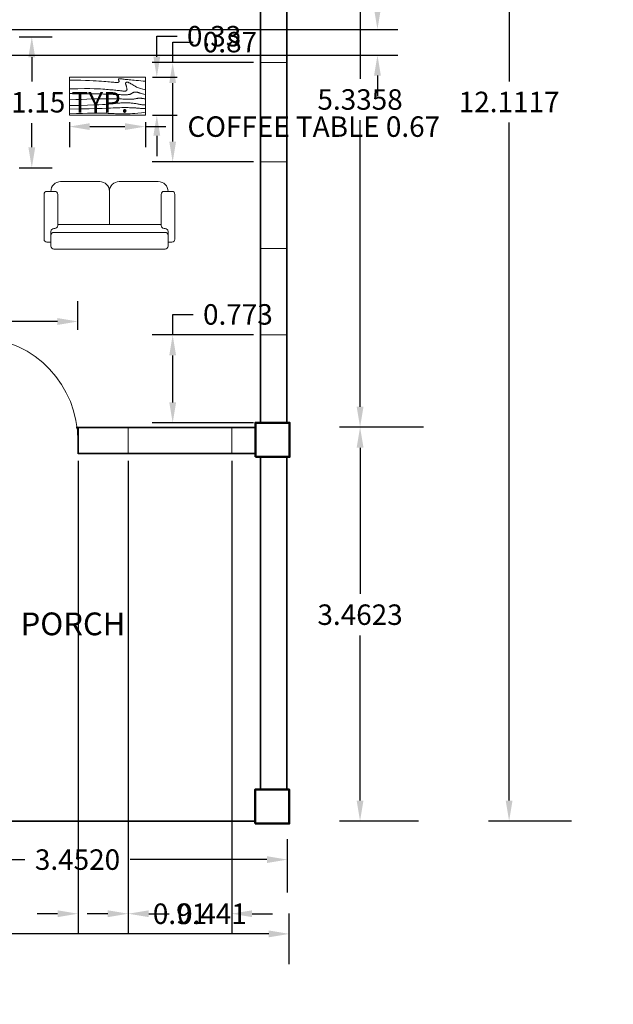
# Model space of a CAD drawing. Units: metres. Extents: x 473.2 to 488.6, y 701.8 to 717.3.
# Tile 3 of 4: x 483.4 to 488.6, y 702.6 to 711.3. Entities that reach past the tile are written whole.
import ezdxf

# ---------------------------------------------------------------- set-up
doc = ezdxf.new("R2010")
doc.units = ezdxf.units.M
doc.header["$PDMODE"] = 32
for name, color, linetype, lineweight in [('A-ANNO-DIMS', 2, 'Continuous', 18), ('A-AREA-IDEN', 7, 'Continuous', 18), ('A-COLS', 7, 'Continuous', 50), ('A-DOOR', 3, 'Continuous', 18), ('A-FURN', 8, 'Continuous', 18), ('A-GLAZ', 4, 'Continuous', 18), ('A-WALL', 7, 'Continuous', 35)]:
    doc.layers.add(name, color=color, linetype=linetype, lineweight=lineweight)
doc.styles.get("Standard").update_dxf_attribs({"font": 'arial.ttf'})
doc.dimstyles.get("Standard").update_dxf_attribs({"dimtxt": 0.18, "dimasz": 0.18, "dimexe": 0.18, "dimexo": 0.0625, "dimgap": 0.09, "dimtad": 0, "dimtih": 1, "dimtoh": 1, "dimdec": 4, "dimzin": 0, "dimdsep": 46, "dimtxsty": 'Standard', "dimcen": 0.09, "dimadec": 0, "dimazin": 0, "dimtfac": 1, "dimtdec": 4, "dimtofl": 0, "dimtmove": 0, "dimatfit": 3, "dimfxl": 1, "dimtolj": 1, "dimtzin": 0, "dimarcsym": 0})

# ---------------------------------------------------------------- blocks, each defined once
blk = doc.blocks.new('A$C02A636C4')
for p, q in [((0.0679, 0.6013), (0.0291, 0.6013)), ((0.0679, 0.6401), (0.0679, 0.6013)), ((0.0679, 0.5334), (0.0679, 0.6013)), ((1.2026, 0.6692), (0.097, 0.6692)), ((1.2317, 0.6401), (1.2317, 0.6013)), ((1.2317, 0.6013), (1.2705, 0.6013)), ((1.2317, 0.5334), (1.2317, 0.6013)), ((0, 0.5722), (0, 0.1261)), ((0.0679, 0.4946), (0.0679, 0.5431)), ((1.2026, 0.5043), (0.097, 0.5043)), ((1.2317, 0.4946), (1.2317, 0.5431)), ((1.2996, 0.5722), (1.2996, 0.1261)), ((0.1067, 0.4655), (0.097, 0.4655)), ((0.1358, 0.1261), (0.1358, 0.4364)), ((1.1638, 0.4267), (0.1358, 0.4267)), ((0.6498, 0.097), (0.6498, 0.4267)), ((1.1638, 0.1261), (1.1638, 0.4364)), ((1.1929, 0.4655), (1.2026, 0.4655)), ((0.0291, 0.097), (0.1067, 0.097)), ((0.1649, 0), (0.5528, 0)), ((0.7468, 0), (1.1347, 0)), ((1.2705, 0.097), (1.1929, 0.097))]:
    blk.add_line(p, q)
for centre, radius, start, end in [((0.0291, 0.5722), 0.0291, 90, 180), ((0.097, 0.6401), 0.0291, 90, 180), ((1.2026, 0.6401), 0.0291, 0, 90), ((1.2705, 0.5722), 0.0291, 0, 90), ((0.097, 0.5334), 0.0291, 180, 270), ((0.097, 0.4946), 0.0291, 180, 270), ((1.2026, 0.5334), 0.0291, 270, 0), ((1.2026, 0.4946), 0.0291, 270, 0), ((0.1067, 0.4364), 0.0291, 0, 90), ((1.1929, 0.4364), 0.0291, 90, 180), ((0.0291, 0.1261), 0.0291, 180, 270), ((0.1067, 0.1261), 0.0291, 270, 0), ((1.1929, 0.1261), 0.0291, 180, 270), ((1.2705, 0.1261), 0.0291, 270, 0), ((0.1649, 0.097), 0.097, 180, 270), ((0.5528, 0.097), 0.097, 270, 0), ((0.7468, 0.097), 0.097, 180, 270), ((1.1347, 0.097), 0.097, 270, 0)]:
    blk.add_arc(centre, radius, start, end)
blk = doc.blocks.new('Table - Rectangular Woodgrain 60 x 30 in.')
for p, q in [((0, 0), (0, -30)), ((60, 0), (0, 0)), ((60, -30), (60, 0)), ((0, -30), (60, -30))]:
    blk.add_line(p, q)
for points in [[(0, -2.4), (4.8155, -2.418), (9.0302, -2.4688), (12.709, -2.5477), (15.9167, -2.65), (18.7181, -2.7711), (21.1781, -2.9063), (23.3616, -3.0508), (25.3333, -3.2), (27.1477, -3.3495), (28.8172, -3.4958), (30.3437, -3.636), (31.7291, -3.7667), (32.9756, -3.8849), (34.0849, -3.9875), (35.059, -4.0714), (35.9, -4.1334), (36.6114, -4.1711), (37.2041, -4.1854), (37.6906, -4.1779), (38.0833, -4.15), (38.3948, -4.1034), (38.6375, -4.0396), (38.8239, -3.9602), (38.9666, -3.8667), (39.0764, -3.7608), (39.1573, -3.6448), (39.2116, -3.521), (39.2416, -3.3917), (39.2498, -3.2593), (39.2385, -3.1261), (39.21, -2.9944), (39.1666, -2.8667), (39.111, -2.7447), (39.0468, -2.6281), (38.978, -2.5163), (38.9083, -2.4083), (38.8418, -2.3035), (38.7823, -2.201), (38.7337, -2.1001), (38.7, -2), (38.6844, -1.9003), (38.6875, -1.8021), (38.7094, -1.707), (38.75, -1.6167), (38.8094, -1.5326), (38.8875, -1.4563), (38.9844, -1.3893), (39.1, -1.3333), (39.2351, -1.2896), (39.3937, -1.2583), (39.5804, -1.2396), (39.8, -1.2333), (40.057, -1.2396), (40.3562, -1.2583), (40.7023, -1.2896), (41.1, -1.3333), (41.5547, -1.3895), (42.0755, -1.4573), (42.6721, -1.5361), (43.3542, -1.625), (44.1316, -1.7233), (45.014, -1.8302), (46.0114, -1.9449), (47.1333, -2.0667), (48.3862, -2.1947), (49.7625, -2.3281), (51.2513, -2.4663), (52.8416, -2.6083), (54.5226, -2.7535), (56.2833, -2.9011), (58.1127, -3.0501), (60, -3.2)], [(0, -9.2), (6.5759, -9.0858), (11.9385, -9.0365), (16.2527, -9.0418), (19.6833, -9.0917), (22.3952, -9.1759), (24.5531, -9.2844), (26.322, -9.4069), (27.8666, -9.5333), (29.3241, -9.6553), (30.7203, -9.7719), (32.0532, -9.8837), (33.3208, -9.9917), (34.5213, -10.0965), (35.6526, -10.199), (36.7128, -10.2999), (37.7, -10.4), (38.6129, -10.4996), (39.4531, -10.5969), (40.223, -10.6895), (40.925, -10.775), (41.5613, -10.8512), (42.1344, -10.9156), (42.6465, -10.966), (43.1, -11), (43.4976, -11.0158), (43.8437, -11.0136), (44.143, -10.9942), (44.4, -10.9583), (44.6195, -10.9069), (44.8062, -10.8406), (44.9648, -10.7603), (45.1, -10.6667), (45.2155, -10.5598), (45.3114, -10.4365), (45.3871, -10.2929), (45.4416, -10.125), (45.4743, -9.929), (45.4844, -9.7011), (45.4709, -9.4371), (45.4333, -9.1333), (45.3716, -8.7883), (45.2896, -8.4104), (45.1919, -8.0107), (45.0833, -7.6), (44.9685, -7.1893), (44.8521, -6.7896), (44.7388, -6.4117), (44.6333, -6.0667), (44.54, -5.7628), (44.4614, -5.4979), (44.4001, -5.2675), (44.3583, -5.0667), (44.3384, -4.8909), (44.3427, -4.7354), (44.3736, -4.5956), (44.4333, -4.4667), (44.5236, -4.3453), (44.6427, -4.2333), (44.7884, -4.1339), (44.9583, -4.05), (45.1501, -3.9849), (45.3614, -3.9417), (45.59, -3.9234), (45.8333, -3.9333), (46.0915, -3.9749), (46.3734, -4.0531), (46.6906, -4.1736), (47.0542, -4.3417), (47.4756, -4.5629), (47.9661, -4.8427), (48.5372, -5.1866), (49.2, -5.6), (49.9676, -6.0844), (50.8594, -6.625), (51.8965, -7.2031), (53.1, -7.8), (54.491, -8.3969), (56.0906, -8.975), (57.9199, -9.5156), (60, -10)], [(0, -12.8), (5.1847, -12.9322), (9.6213, -13.0323), (13.3963, -13.1059), (16.5958, -13.1583), (19.3063, -13.1952), (21.614, -13.2219), (23.6054, -13.2439), (25.3666, -13.2667), (26.9728, -13.2947), (28.4531, -13.3281), (29.8256, -13.3663), (31.1083, -13.4083), (32.3191, -13.4535), (33.476, -13.501), (34.597, -13.5501), (35.7, -13.6), (36.7984, -13.6497), (37.8875, -13.6979), (38.9578, -13.743), (40, -13.7833), (41.0047, -13.8174), (41.9625, -13.8438), (42.864, -13.8607), (43.7, -13.8667), (44.4631, -13.8604), (45.1552, -13.8417), (45.7801, -13.8104), (46.3416, -13.7667), (46.8439, -13.7104), (47.2906, -13.6417), (47.6858, -13.5604), (48.0333, -13.4667), (48.3375, -13.3608), (48.6042, -13.2448), (48.8396, -13.121), (49.05, -12.9917), (49.2417, -12.8593), (49.4208, -12.7261), (49.5937, -12.5944), (49.7667, -12.4667), (49.9452, -12.3451), (50.1323, -12.2313), (50.3303, -12.1268), (50.5416, -12.0333), (50.7686, -11.9524), (51.0135, -11.8854), (51.2788, -11.8341), (51.5666, -11.8), (51.8785, -11.7843), (52.2116, -11.7865), (52.562, -11.8059), (52.926, -11.8417), (53.2998, -11.8931), (53.6795, -11.9594), (54.0614, -12.0397), (54.4416, -12.1333), (54.8223, -12.2401), (55.2293, -12.3625), (55.6942, -12.5037), (56.2489, -12.6667), (56.9251, -12.8547), (57.7545, -13.0708), (58.7689, -13.3182), (60, -13.6)], [(0, -18), (5.124, -17.7273), (9.6609, -17.5057), (13.6705, -17.3303), (17.2125, -17.1958), (20.3467, -17.0973), (23.1328, -17.0297), (25.6307, -16.9878), (27.9, -16.9667), (29.9928, -16.9617), (31.9302, -16.9703), (33.7254, -16.9907), (35.3917, -17.0208), (36.9423, -17.0588), (38.3906, -17.1026), (39.7499, -17.1503), (41.0333, -17.2), (42.2519, -17.2496), (43.4073, -17.2969), (44.4986, -17.3395), (45.525, -17.375), (46.4858, -17.4012), (47.3802, -17.4156), (48.2074, -17.416), (48.9667, -17.4), (49.6583, -17.3662), (50.2872, -17.3167), (50.8595, -17.2547), (51.3812, -17.1833), (51.8584, -17.1057), (52.2971, -17.025), (52.7034, -16.9443), (53.0833, -16.8667), (53.443, -16.7951), (53.789, -16.7313), (54.128, -16.6768), (54.4666, -16.6334), (54.8115, -16.6024), (55.1693, -16.5854), (55.5465, -16.5841), (55.95, -16.6), (56.3828, -16.6337), (56.8346, -16.6823), (57.2915, -16.7418), (57.7396, -16.8084), (58.165, -16.878), (58.5539, -16.9469), (58.8924, -17.0111), (59.1666, -17.0667), (59.3679, -17.1107), (59.5078, -17.1438), (59.6032, -17.1675), (59.6708, -17.1833), (59.7275, -17.193), (59.7901, -17.1979), (59.8753, -17.1998), (60, -17.2)], [(0, -22.4), (8.0098, -22.2501), (14.4094, -22.1011), (19.4168, -21.9535), (23.25, -21.8083), (26.1269, -21.6663), (28.2656, -21.5281), (29.884, -21.3947), (31.2, -21.2667), (32.3967, -21.1448), (33.5172, -21.0292), (34.5697, -20.9198), (35.5625, -20.8167), (36.5037, -20.7198), (37.4015, -20.6292), (38.2642, -20.5448), (39.1, -20.4667), (39.9164, -20.3951), (40.7187, -20.3313), (41.5117, -20.2768), (42.3, -20.2333), (43.0883, -20.2024), (43.8812, -20.1854), (44.6836, -20.1841), (45.5, -20.2), (46.3328, -20.234), (47.1747, -20.2844), (48.0163, -20.3488), (48.8479, -20.425), (49.66, -20.5106), (50.4429, -20.6031), (51.1872, -20.7004), (51.8833, -20.8), (52.5246, -20.8999), (53.1166, -20.9995), (53.6681, -21.0983), (54.1875, -21.1958), (54.6834, -21.2919), (55.1646, -21.3859), (55.6394, -21.4777), (56.1167, -21.5667), (56.6028, -21.6515), (57.0961, -21.7266), (57.5929, -21.7852), (58.0896, -21.8208), (58.5823, -21.8268), (59.0674, -21.7964), (59.5412, -21.723), (60, -21.6)], [(0, -25.2), (8.6355, -25.0504), (15.7026, -24.9031), (21.4049, -24.7606), (25.9458, -24.625), (29.529, -24.4988), (32.3578, -24.3844), (34.6359, -24.284), (36.5667, -24.2), (38.3213, -24.1341), (39.9417, -24.0854), (41.437, -24.0523), (42.8167, -24.0333), (44.0901, -24.0268), (45.2667, -24.0313), (46.3557, -24.0451), (47.3667, -24.0667), (48.309, -24.0947), (49.1928, -24.1287), (50.0284, -24.168), (50.826, -24.2125), (51.5959, -24.2617), (52.3483, -24.3151), (53.0935, -24.3725), (53.8417, -24.4334), (54.6009, -24.497), (55.3699, -24.561), (56.1454, -24.6226), (56.9239, -24.6792), (57.7021, -24.7279), (58.4764, -24.7662), (59.2435, -24.7911), (60, -24.8)], [(0, -28.8), (5.6867, -28.6681), (10.45, -28.5698), (14.407, -28.5012), (17.675, -28.4584), (20.3711, -28.4374), (22.6125, -28.4344), (24.5164, -28.4455), (26.2, -28.4667), (27.762, -28.4947), (29.2276, -28.5281), (30.6033, -28.5663), (31.8958, -28.6084), (33.1118, -28.6535), (34.2578, -28.7011), (35.3405, -28.7501), (36.3666, -28.8), (37.3443, -28.8497), (38.288, -28.8974), (39.2137, -28.9412), (40.1375, -28.9792), (41.0753, -29.0093), (42.0432, -29.0297), (43.0572, -29.0384), (44.1333, -29.0333), (45.2936, -29.0114), (46.5843, -28.9641), (48.0579, -28.8816), (49.7666, -28.7542), (51.7629, -28.5721), (54.0989, -28.3255), (56.8272, -28.0048), (60, -27.6)]]:
    blk.add_lwpolyline(points)
blk = doc.blocks.new('*D14')
at = {"layer": 'A-ANNO-DIMS', "color": 0, "lineweight": -2, "transparency": 16777216}
for p, q in [((486.6804, 713.0126), (486.1829, 713.0126)), ((486.3629, 712.8326), (486.3629, 710.7399)), ((486.3629, 707.8568), (486.3629, 710.376)), ((486.9196, 707.6768), (486.1829, 707.6768))]:
    blk.add_line(p, q, dxfattribs=at)
at = {"layer": 'A-ANNO-DIMS', "color": 0, "transparency": 16777216}
for points in [[(486.3329, 712.8326), (486.3929, 712.8326), (486.3629, 713.0126)], [(486.3329, 707.8568), (486.3929, 707.8568), (486.3629, 707.6768)]]:
    blk.add_solid(points, dxfattribs=at)
at = {"layer": 'Defpoints', "color": 0, "transparency": 16777216}
for p in [(486.3629, 713.0126), (486.7429, 713.0126), (486.9821, 707.6768)]:
    blk.add_point(p, dxfattribs=at)
at = {"layer": 'A-ANNO-DIMS', "color": 0, "transparency": 16777216, "insert": (486.3629, 710.5579), "char_height": 0.18, "width": 1.240263, "attachment_point": 5}
blk.add_mtext('\\A1;5.3358', dxfattribs=at)
blk = doc.blocks.new('*D15')
at = {"layer": 'A-ANNO-DIMS', "color": 0, "lineweight": -2, "transparency": 16777216}
for p, q in [((486.5856, 707.6768), (486.1829, 707.6768)), ((486.3629, 707.4968), (486.3629, 706.2104)), ((486.3629, 704.3946), (486.3629, 705.8465)), ((486.877, 704.2146), (486.1829, 704.2146))]:
    blk.add_line(p, q, dxfattribs=at)
at = {"layer": 'A-ANNO-DIMS', "color": 0, "transparency": 16777216}
for points in [[(486.3329, 707.4968), (486.3929, 707.4968), (486.3629, 707.6768)], [(486.3329, 704.3946), (486.3929, 704.3946), (486.3629, 704.2146)]]:
    blk.add_solid(points, dxfattribs=at)
at = {"layer": 'Defpoints', "color": 0, "transparency": 16777216}
for p in [(486.3629, 707.6768), (486.6481, 707.6768), (486.9395, 704.2146)]:
    blk.add_point(p, dxfattribs=at)
at = {"layer": 'A-ANNO-DIMS', "color": 0, "transparency": 16777216, "insert": (486.3629, 706.0285), "char_height": 0.18, "width": 1.240263, "attachment_point": 5}
blk.add_mtext('\\A1;3.4623', dxfattribs=at)
blk = doc.blocks.new('*D17')
at = {"layer": 'A-ANNO-DIMS', "color": 0, "lineweight": -2, "transparency": 16777216}
for p, q in [((488.5274, 716.3262), (487.4937, 716.3262)), ((487.6737, 716.1462), (487.6737, 710.7165)), ((487.6737, 704.3946), (487.6737, 710.3558)), ((488.2227, 704.2146), (487.4937, 704.2146))]:
    blk.add_line(p, q, dxfattribs=at)
at = {"layer": 'A-ANNO-DIMS', "color": 0, "transparency": 16777216}
for points in [[(487.6437, 716.1462), (487.7037, 716.1462), (487.6737, 716.3262)], [(487.6437, 704.3946), (487.7037, 704.3946), (487.6737, 704.2146)]]:
    blk.add_solid(points, dxfattribs=at)
at = {"layer": 'Defpoints', "color": 0, "transparency": 16777216}
for p in [(487.6737, 716.3262), (488.5899, 716.3262), (488.2852, 704.2146)]:
    blk.add_point(p, dxfattribs=at)
at = {"layer": 'A-ANNO-DIMS', "color": 0, "transparency": 16777216, "insert": (487.6737, 710.5362), "char_height": 0.18, "width": 1.240263, "attachment_point": 5}
blk.add_mtext('\\A1;12.1117', dxfattribs=at)
blk = doc.blocks.new('*D18')
at = {"layer": 'A-ANNO-DIMS', "color": 0, "lineweight": -2, "transparency": 16777216}
for p, q in [((475.798, 702.6656), (475.798, 703.4022)), ((485.74, 702.957), (485.74, 703.4022)), ((475.978, 703.2222), (480.3782, 703.2222)), ((485.56, 703.2222), (481.3049, 703.2222))]:
    blk.add_line(p, q, dxfattribs=at)
at = {"layer": 'A-ANNO-DIMS', "color": 0, "transparency": 16777216}
for points in [[(475.978, 703.2522), (475.978, 703.1922), (475.798, 703.2222)], [(485.56, 703.2522), (485.56, 703.1922), (485.74, 703.2222)]]:
    blk.add_solid(points, dxfattribs=at)
at = {"layer": 'Defpoints', "color": 0, "transparency": 16777216}
for p in [(485.74, 703.2222), (485.74, 702.8945), (475.798, 702.6031)]:
    blk.add_point(p, dxfattribs=at)
at = {"layer": 'A-ANNO-DIMS', "color": 0, "transparency": 16777216, "insert": (480.8416, 703.2222), "char_height": 0.18, "width": 1.240263, "attachment_point": 5}
blk.add_mtext('\\A1;9.9420', dxfattribs=at)
blk = doc.blocks.new('*D21')
at = {"layer": 'A-ANNO-DIMS', "color": 0, "lineweight": -2, "transparency": 16777216}
for p, q in [((482.2714, 703.3187), (482.2714, 704.0553)), ((485.7234, 703.5853), (485.7234, 704.0553)), ((482.4514, 703.8753), (483.415, 703.8753)), ((485.5434, 703.8753), (484.3415, 703.8753))]:
    blk.add_line(p, q, dxfattribs=at)
at = {"layer": 'A-ANNO-DIMS', "color": 0, "transparency": 16777216}
for points in [[(482.4514, 703.9053), (482.4514, 703.8453), (482.2714, 703.8753)], [(485.5434, 703.9053), (485.5434, 703.8453), (485.7234, 703.8753)]]:
    blk.add_solid(points, dxfattribs=at)
at = {"layer": 'Defpoints', "color": 0, "transparency": 16777216}
for p in [(485.7234, 703.8753), (485.7234, 703.5228), (482.2714, 703.2562)]:
    blk.add_point(p, dxfattribs=at)
at = {"layer": 'A-ANNO-DIMS', "color": 0, "transparency": 16777216, "insert": (483.8782, 703.8753), "char_height": 0.18, "width": 1.240263, "attachment_point": 5}
blk.add_mtext('\\A1;3.4520', dxfattribs=at)
blk = doc.blocks.new('DOOR-SWING-910')
for p, q in [((0, 0), (-0.05, 0)), ((-0.05, 0), (-0.05, -0.91)), ((0, 0), (0, -0.91)), ((0, -0.91), (-0.05, -0.91))]:
    blk.add_line(p, q)
blk.add_arc((0.0015, 0), 0.9115, 180, 266.76381)
blk = doc.blocks.new('COL-SQUARE-300')
blk.add_lwpolyline([(-0.15, -0.15), (0.15, -0.15), (0.15, 0.15), (-0.15, 0.15)], close=True)
blk = doc.blocks.new('WIN-1520')
blk.add_line((0.23, 0.76), (0, 0.76))
blk.add_lwpolyline([(0.23, 0), (0.23, 1.52), (0, 1.52), (0, 0)], close=True)
blk = doc.blocks.new('*D27')
at = {"layer": 'A-ANNO-DIMS', "color": 0, "lineweight": -2, "transparency": 16777216}
for p, q in [((482.9717, 708.5321), (482.9717, 708.7861)), ((483.8817, 708.5321), (483.8817, 708.7861)), ((482.9717, 708.6061), (482.7917, 708.6061)), ((483.7017, 708.6061), (483.1517, 708.6061))]:
    blk.add_line(p, q, dxfattribs=at)
at = {"layer": 'A-ANNO-DIMS', "color": 0, "transparency": 16777216}
for points in [[(483.1517, 708.6361), (483.1517, 708.5761), (482.9717, 708.6061)], [(483.7017, 708.6361), (483.7017, 708.5761), (483.8817, 708.6061)]]:
    blk.add_solid(points, dxfattribs=at)
at = {"layer": 'Defpoints', "color": 0, "transparency": 16777216}
for p in [(482.9717, 708.6061), (482.9717, 708.4696), (483.8817, 708.4696)]:
    blk.add_point(p, dxfattribs=at)
at = {"layer": 'A-ANNO-DIMS', "color": 0, "transparency": 16777216, "insert": (481.7511, 708.6061), "char_height": 0.18, "attachment_point": 5}
blk.add_mtext('\\A1;DOOR 0.91 TYP.', dxfattribs=at)
blk = doc.blocks.new('*D33')
at = {"layer": 'A-ANNO-DIMS', "color": 0, "lineweight": -2, "transparency": 16777216}
for p, q in [((483.3662, 711.1086), (483.6562, 711.1086)), ((483.4762, 710.9286), (483.4762, 710.7165)), ((483.4762, 710.1382), (483.4762, 710.3503)), ((483.3662, 709.9582), (483.6562, 709.9582))]:
    blk.add_line(p, q, dxfattribs=at)
at = {"layer": 'A-ANNO-DIMS', "color": 0, "transparency": 16777216}
for points in [[(483.4462, 710.9286), (483.5062, 710.9286), (483.4762, 711.1086)], [(483.4462, 710.1382), (483.5062, 710.1382), (483.4762, 709.9582)]]:
    blk.add_solid(points, dxfattribs=at)
at = {"layer": 'Defpoints', "color": 0, "transparency": 16777216}
for p in [(483.3037, 711.1086), (483.3037, 709.9582), (483.4762, 709.9582)]:
    blk.add_point(p, dxfattribs=at)
at = {"layer": 'A-ANNO-DIMS', "color": 0, "transparency": 16777216, "insert": (483.4762, 710.5334), "char_height": 0.18, "attachment_point": 5}
blk.add_mtext('\\A1;SOFA 1.15 TYP.', dxfattribs=at)
blk = doc.blocks.new('*D35')
at = {"layer": 'A-ANNO-DIMS', "color": 0, "lineweight": -2, "transparency": 16777216}
for p, q in [((483.8064, 710.3573), (483.8064, 710.1394)), ((484.4752, 710.3573), (484.4752, 710.1394)), ((483.9864, 710.3194), (484.2952, 710.3194)), ((484.4752, 710.3194), (484.6552, 710.3194))]:
    blk.add_line(p, q, dxfattribs=at)
at = {"layer": 'A-ANNO-DIMS', "color": 0, "transparency": 16777216}
for points in [[(483.9864, 710.3494), (483.9864, 710.2894), (483.8064, 710.3194)], [(484.2952, 710.3494), (484.2952, 710.2894), (484.4752, 710.3194)]]:
    blk.add_solid(points, dxfattribs=at)
at = {"layer": 'Defpoints', "color": 0, "transparency": 16777216}
for p in [(483.8064, 710.4198), (484.4752, 710.4198), (484.4752, 710.3194)]:
    blk.add_point(p, dxfattribs=at)
at = {"layer": 'A-ANNO-DIMS', "color": 0, "transparency": 16777216, "insert": (485.956, 710.3194), "char_height": 0.18, "attachment_point": 5}
blk.add_mtext('\\A1;COFFEE TABLE 0.67', dxfattribs=at)
blk = doc.blocks.new('*D36')
at = {"layer": 'A-ANNO-DIMS', "color": 0, "lineweight": -2, "transparency": 16777216}
for p, q in [((484.5755, 710.9342), (484.5755, 711.1142)), ((484.5755, 711.1142), (484.7555, 711.1142)), ((484.5377, 710.7542), (484.7555, 710.7542)), ((484.5377, 710.4198), (484.7555, 710.4198)), ((484.5755, 710.2398), (484.5755, 710.0598))]:
    blk.add_line(p, q, dxfattribs=at)
at = {"layer": 'A-ANNO-DIMS', "color": 0, "transparency": 16777216}
for points in [[(484.5455, 710.9342), (484.6055, 710.9342), (484.5755, 710.7542)], [(484.5455, 710.2398), (484.6055, 710.2398), (484.5755, 710.4198)]]:
    blk.add_solid(points, dxfattribs=at)
at = {"layer": 'Defpoints', "color": 0, "transparency": 16777216}
for p in [(484.4752, 710.7542), (484.5755, 710.7542), (484.4752, 710.4198)]:
    blk.add_point(p, dxfattribs=at)
at = {"layer": 'A-ANNO-DIMS', "color": 0, "transparency": 16777216, "insert": (485.0793, 711.1142), "char_height": 0.18, "attachment_point": 5}
blk.add_mtext('\\A1;0.33', dxfattribs=at)
blk = doc.blocks.new('*D44')
at = {"layer": 'A-ANNO-DIMS', "color": 0, "lineweight": -2, "transparency": 16777216}
for p, q in [((486.5158, 711.3546), (486.5158, 711.5346)), ((486.5158, 711.5346), (486.6958, 711.5346)), ((478.5905, 711.1746), (486.6958, 711.1746)), ((478.5905, 710.9478), (486.6958, 710.9478)), ((486.5158, 710.7678), (486.5158, 710.5878))]:
    blk.add_line(p, q, dxfattribs=at)
at = {"layer": 'A-ANNO-DIMS', "color": 0, "transparency": 16777216}
for points in [[(486.4858, 711.3546), (486.5458, 711.3546), (486.5158, 711.1746)], [(486.4858, 710.7678), (486.5458, 710.7678), (486.5158, 710.9478)]]:
    blk.add_solid(points, dxfattribs=at)
at = {"layer": 'Defpoints', "color": 0, "transparency": 16777216}
for p in [(478.528, 711.1746), (486.5158, 711.1746), (478.528, 710.9478)]:
    blk.add_point(p, dxfattribs=at)
at = {"layer": 'A-ANNO-DIMS', "color": 0, "transparency": 16777216, "insert": (487.0196, 711.5346), "char_height": 0.18, "attachment_point": 5}
blk.add_mtext('\\A1;0.23', dxfattribs=at)
blk = doc.blocks.new('*D56')
at = {"layer": 'A-ANNO-DIMS', "color": 0, "lineweight": -2, "transparency": 16777216}
for p, q in [((484.715, 708.4883), (484.715, 708.6683)), ((484.715, 708.6683), (484.895, 708.6683)), ((485.4255, 708.4883), (484.535, 708.4883)), ((484.715, 707.8953), (484.715, 708.3083)), ((485.4255, 707.7153), (484.535, 707.7153))]:
    blk.add_line(p, q, dxfattribs=at)
at = {"layer": 'A-ANNO-DIMS', "color": 0, "transparency": 16777216}
for points in [[(484.685, 708.3083), (484.745, 708.3083), (484.715, 708.4883)], [(484.685, 707.8953), (484.745, 707.8953), (484.715, 707.7153)]]:
    blk.add_solid(points, dxfattribs=at)
at = {"layer": 'Defpoints', "color": 0, "transparency": 16777216}
for p in [(484.715, 708.4883), (485.488, 708.4883), (485.488, 707.7153)]:
    blk.add_point(p, dxfattribs=at)
at = {"layer": 'A-ANNO-DIMS', "color": 0, "transparency": 16777216, "insert": (485.2887, 708.6683), "char_height": 0.18, "attachment_point": 5}
blk.add_mtext('\\A1;0.773', dxfattribs=at)
blk = doc.blocks.new('*D57')
at = {"layer": 'A-ANNO-DIMS', "color": 0, "lineweight": -2, "transparency": 16777216}
for p, q in [((484.715, 710.8821), (484.715, 711.0621)), ((484.715, 711.0621), (484.895, 711.0621)), ((485.4255, 710.8821), (484.535, 710.8821)), ((484.715, 710.1883), (484.715, 710.7021)), ((485.4255, 710.0083), (484.535, 710.0083))]:
    blk.add_line(p, q, dxfattribs=at)
at = {"layer": 'A-ANNO-DIMS', "color": 0, "transparency": 16777216}
for points in [[(484.685, 710.7021), (484.745, 710.7021), (484.715, 710.8821)], [(484.685, 710.1883), (484.745, 710.1883), (484.715, 710.0083)]]:
    blk.add_solid(points, dxfattribs=at)
at = {"layer": 'Defpoints', "color": 0, "transparency": 16777216}
for p in [(484.715, 710.8821), (485.488, 710.8821), (485.488, 710.0083)]:
    blk.add_point(p, dxfattribs=at)
at = {"layer": 'A-ANNO-DIMS', "color": 0, "transparency": 16777216, "insert": (485.2187, 711.0621), "char_height": 0.18, "attachment_point": 5}
blk.add_mtext('\\A1;0.87', dxfattribs=at)
blk = doc.blocks.new('*D62')
at = {"layer": 'A-ANNO-DIMS', "color": 0, "lineweight": -2, "transparency": 16777216}
for p, q in [((484.324028, 707.382057), (484.324028, 703.219503)), ((485.234028, 707.382057), (485.234028, 703.219503)), ((484.144028, 703.399503), (483.964028, 703.399503)), ((485.414028, 703.399503), (485.594028, 703.399503))]:
    blk.add_line(p, q, dxfattribs=at)
at = {"layer": 'A-ANNO-DIMS', "color": 0, "transparency": 16777216}
for points in [[(484.144028, 703.429503), (484.144028, 703.369503), (484.324028, 703.399503)], [(485.414028, 703.429503), (485.414028, 703.369503), (485.234028, 703.399503)]]:
    blk.add_solid(points, dxfattribs=at)
at = {"layer": 'Defpoints', "color": 0, "transparency": 16777216}
for p in [(484.324028, 707.444557), (485.234028, 707.444557), (485.234028, 703.399503)]:
    blk.add_point(p, dxfattribs=at)
at = {"layer": 'A-ANNO-DIMS', "color": 0, "transparency": 16777216, "insert": (484.779028, 703.399503), "char_height": 0.18, "attachment_point": 5}
blk.add_mtext('\\A1;0.91', dxfattribs=at)
blk = doc.blocks.new('*D63')
at = {"layer": 'A-ANNO-DIMS', "color": 0, "lineweight": -2, "transparency": 16777216}
for p, q in [((483.883, 707.3806), (483.883, 703.2195)), ((484.324, 707.3821), (484.324, 703.2195)), ((483.703, 703.3995), (483.523, 703.3995)), ((484.504, 703.3995), (484.684, 703.3995))]:
    blk.add_line(p, q, dxfattribs=at)
at = {"layer": 'A-ANNO-DIMS', "color": 0, "transparency": 16777216}
for points in [[(483.703, 703.4295), (483.703, 703.3695), (483.883, 703.3995)], [(484.504, 703.4295), (484.504, 703.3695), (484.324, 703.3995)]]:
    blk.add_solid(points, dxfattribs=at)
at = {"layer": 'Defpoints', "color": 0, "transparency": 16777216}
for p in [(483.883, 707.4431), (484.324, 707.4446), (484.324, 703.3995)]:
    blk.add_point(p, dxfattribs=at)
at = {"layer": 'A-ANNO-DIMS', "color": 0, "transparency": 16777216, "insert": (485.0604, 703.3995), "char_height": 0.18, "attachment_point": 5}
blk.add_mtext('\\A1;0.441', dxfattribs=at)

msp = doc.modelspace()

# ---------------------------------------------------------------- linework, layer by layer
at = {"layer": 'A-GLAZ'}
msp.add_lwpolyline([(485.23403, 707.67456), (484.32403, 707.67456), (484.32403, 707.44456), (485.23403, 707.44456)], close=True, dxfattribs=at)
at = {"layer": 'A-WALL'}
for p, q in [((485.48797, 707.71527), (485.48797, 712.85771)), ((485.71797, 707.71527), (485.71797, 712.85771)), ((483.86699, 707.67456), (485.44284, 707.67456)), ((483.88302, 707.44313), (483.88302, 707.67313)), ((483.88302, 707.44456), (484.07527, 707.44456)), ((484.07527, 707.44456), (485.44284, 707.44456)), ((485.48797, 704.49124), (485.48797, 707.41527)), ((485.71797, 704.49124), (485.71797, 707.41527)), ((482.51829, 704.21456), (485.43996, 704.21456))]:
    msp.add_line(p, q, dxfattribs=at)

# ---------------------------------------------------------------- block references
at = {"layer": 'A-COLS'}
for p in [(485.59284, 707.56527), (485.58996, 704.34124)]:
    msp.add_blockref('COL-SQUARE-300', p, dxfattribs=at)
at = {"layer": 'A-DOOR', "rotation": 180}
msp.add_blockref('DOOR-SWING-910', (482.97169, 707.55956), dxfattribs=at)
at = {"layer": 'A-FURN', "xscale": 0.01114641790596, "yscale": 0.01114641790596, "zscale": 0.01114641790596}
msp.add_blockref('Table - Rectangular Woodgrain 60 x 30 in.', (483.80639, 710.75415), dxfattribs=at)
at = {"layer": 'A-FURN', "xscale": -0.8851373679523337, "yscale": 0.8851373679523337, "zscale": 0.8851373679523337, "rotation": 180}
msp.add_blockref('A$C02A636C4', (483.58388, 709.83556), dxfattribs=at)
at = {"layer": 'A-GLAZ'}
for p in [(485.48797, 710.88205), (485.48797, 708.48832)]:
    msp.add_blockref('WIN-1520', p, dxfattribs=at)

# ---------------------------------------------------------------- texts
at = {"layer": 'A-AREA-IDEN', "insert": (483.37775, 706.04762), "char_height": 0.2, "attachment_point": 1}
msp.add_mtext_dynamic_manual_height_columns('PORCH', width=2.8211562, gutter_width=12.5, heights=[0], dxfattribs=at)

# ---------------------------------------------------------------- dimensions: what is measured, and where the dimension line sits
at = {"layer": 'A-ANNO-DIMS'}
for base, p1, p2, picture, middle in [((487.67367, 716.32625), (488.28524, 704.21456), (488.58994, 716.32625), '*D17', (487.67367, 710.53618)), ((486.36295, 713.01265), (486.98209, 707.67682), (486.74295, 713.01265), '*D14', (486.36295, 710.55792)), ((486.36295, 707.67682), (486.93947, 704.21456), (486.64807, 707.67682), '*D15', (486.36295, 706.02846))]:
    dim = msp.add_linear_dim(base=base, p1=p1, p2=p2, angle=90, dimstyle='Standard', override={"dimclrd": 0, "dimclre": 0, "dimclrt": 0}, dxfattribs=at)
    dim.commit()
    dim.dimension.update_dxf_attribs({"geometry": picture, "text_midpoint": middle, "dimtype": 160})
for base, p1, p2, override, picture, middle in [((486.51584, 711.17456), (478.52797, 710.94776), (478.52797, 711.17456), {"dimdec": 2, "dimlfac": 1, "dimrnd": 0, "dimzin": 0, "dimdsep": 46, "dimlunit": 2}, '*D44', (487.01962, 711.53456)), ((484.57549, 710.75415), (484.47517, 710.41976), (484.47517, 710.75415), {"dimdec": 2, "dimlfac": 1, "dimrnd": 0, "dimzin": 0, "dimdsep": 46, "dimlunit": 2}, '*D36', (485.07927, 711.11415)), ((484.71497, 710.88205), (485.48797, 710.00832), (485.48797, 710.88205), {"dimdec": 2, "dimlfac": 1, "dimrnd": 0, "dimzin": 0, "dimdsep": 46, "dimlunit": 2}, '*D57', (485.21875, 711.06205)), ((484.71497, 708.48832), (485.48797, 707.71527), (485.48797, 708.48832), {"dimdec": 3, "dimlfac": 1, "dimrnd": 0, "dimzin": 0, "dimdsep": 46, "dimlunit": 2}, '*D56', (485.28867, 708.66832))]:
    dim = msp.add_linear_dim(base=base, p1=p1, p2=p2, angle=90, dimstyle='Standard', override=override, dxfattribs=at)
    dim.commit()
    dim.dimension.update_dxf_attribs({"geometry": picture, "text_midpoint": middle})
for base, p1, p2, angle, text, picture, middle in [((483.4762, 709.95822), (483.30365, 711.10856), (483.30365, 709.95822), 270, 'SOFA <> TYP.', '*D33', (483.4762, 710.53339)), ((482.97169, 708.60606), (483.88169, 708.46956), (482.97169, 708.46956), 180, 'DOOR <> TYP.', '*D27', (481.7511, 708.60606))]:
    dim = msp.add_linear_dim(base=base, p1=p1, p2=p2, angle=angle, text=text, dimstyle='Standard', override={"dimdec": 2, "dimlfac": 1, "dimrnd": 0, "dimzin": 0, "dimdsep": 46, "dimlunit": 2}, dxfattribs=at)
    dim.commit()
    dim.dimension.update_dxf_attribs({"geometry": picture, "text_midpoint": middle})
dim = msp.add_linear_dim(base=(484.47517, 710.31944), p1=(483.80639, 710.41976), p2=(484.47517, 710.41976), text='COFFEE TABLE <>', dimstyle='Standard', override={"dimdec": 2, "dimlfac": 1, "dimrnd": 0, "dimzin": 0, "dimdsep": 46, "dimlunit": 2}, dxfattribs=at)
dim.commit()
dim.dimension.update_dxf_attribs({"geometry": '*D35', "text_midpoint": (485.956, 710.31944)})
for base, p1, p2, override, picture, middle in [((484.32403, 703.3995), (483.88302, 707.44313), (484.32403, 707.44456), {"dimdec": 3, "dimlfac": 1, "dimrnd": 0, "dimzin": 0, "dimdsep": 46, "dimlunit": 2}, '*D63', (485.06036, 703.3995)), ((485.23403, 703.3995), (484.32403, 707.44456), (485.23403, 707.44456), {"dimdec": 2, "dimlfac": 1, "dimrnd": 0, "dimzin": 0, "dimdsep": 46, "dimlunit": 2}, '*D62', (484.77903, 703.3995))]:
    dim = msp.add_linear_dim(base=base, p1=p1, p2=p2, dimstyle='Standard', override=override, dxfattribs=at)
    dim.commit()
    dim.dimension.update_dxf_attribs({"geometry": picture, "text_midpoint": middle})
for base, p1, p2, picture, middle in [((485.72339, 703.87534), (482.27142, 703.25619), (485.72339, 703.52275), '*D21', (483.87823, 703.87534)), ((485.73996, 703.22224), (475.79797, 702.6031), (485.73996, 702.8945), '*D18', (480.84155, 703.22224))]:
    dim = msp.add_linear_dim(base=base, p1=p1, p2=p2, dimstyle='Standard', override={"dimclrd": 0, "dimclre": 0, "dimclrt": 0}, dxfattribs=at)
    dim.commit()
    dim.dimension.update_dxf_attribs({"geometry": picture, "text_midpoint": middle, "dimtype": 160})

doc.saveas('drawing.dxf')
